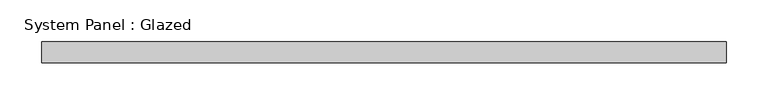
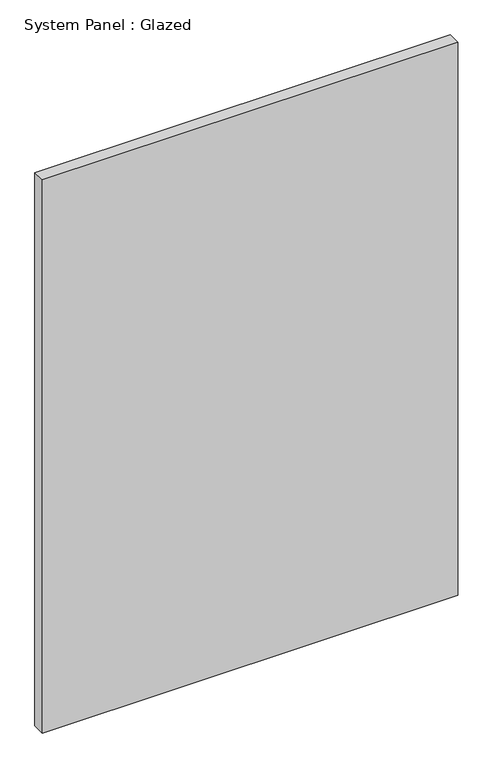
"""IFC4 building model written with IfcOpenShell, lengths in millimetres: plate geometry, System Panel : Glazed."""

from ifc_helpers import new_model, si_unit, origin, origin_with_axes, place, context, project, spatial, polyline, outline, extrude, source, transform, mapped, element, save


def system_panel_glazed_b08a8559(model_context):
    return source(origin(), model_context, "Body", "SweptSolid", [
        extrude(outline(polyline([(410.6082878, 19.05), (-410.6082878, 19.05), (-410.6082878, 44.45), (410.6082878, 44.45), (410.6082878, 19.05)])), origin_with_axes(), (0.0, 0.0, 1.0), 1155.7),
    ])


if __name__ == "__main__":
    model = new_model("IFC4")
    model_context = context("Model", 3, world=origin())
    ifc_project = project(units=[si_unit("LENGTHUNIT", "METRE", prefix="MILLI")], contexts=[model_context])
    site = spatial("IfcSite", under=ifc_project)
    building = spatial("IfcBuilding", under=site)
    placement = place(None, origin())
    system_panel_glazed_shape = system_panel_glazed_b08a8559(model_context)
    element("IfcPlate", 1, ObjectType="System Panel : Glazed", at=placement, inside=building, context=model_context, shape_type="MappedRepresentation", body=[
        mapped(system_panel_glazed_shape, transform((0.0, 0.0, 0.0), x_axis=(1.0, 0.0, 0.0), y_axis=(0.0, 1.0, 0.0), z_axis=(0.0, 0.0, 1.0))),
    ])
    save(model, "model.ifc")

# Revit data of these elements
# Type "System Panel : Glazed"
#   Construction Type Id = "GSP4R"
#   Analytic Construction = "1/8 in Pilkington single glazing"
#   Visual Light Transmittance = 0.9
#   Solar Heat Gain Coefficient = 0.86
#   Heat Transfer Coefficient (U) = 1.18115 BTU/(h·ft²·°F)
# Element 1 (IfcPlate, "System Panel : Glazed")
#   Materials on its faces: "Glass"
# Materials
#   "Glass": class "Glass", colour RGB 0 128 192, transparency 0.75, Description = "Soda Lime Glass", Cost = 0
